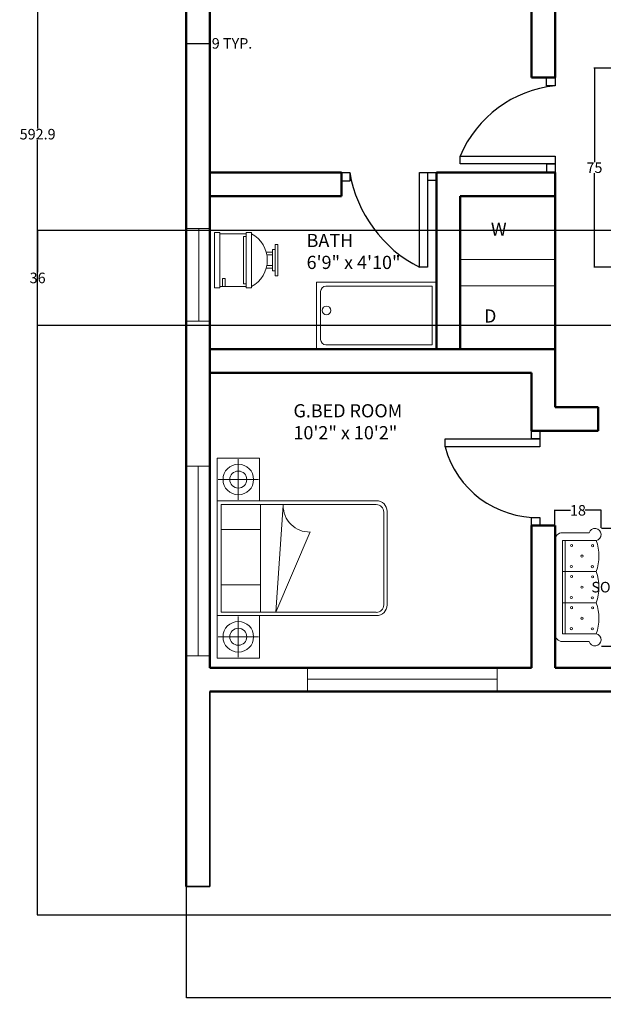
# Model space of a CAD drawing. Units: inches. Extents: x 870 to 1431, y 383 to 1070.
# Tile 1 of 9: x 870 to 1091, y 383 to 756. Entities that reach past the tile are written whole.
import ezdxf

# ---------------------------------------------------------------- set-up
doc = ezdxf.new("R2010")
doc.units = ezdxf.units.IN
doc.header["$MEASUREMENT"] = 0
for name, color, linetype, lineweight in [('A-ANNO-DIMS', 2, 'Continuous', 18), ('A-ANNO-TEXT', 7, 'Continuous', 18), ('A-AREA-IDEN', 7, 'Continuous', 25), ('A-DOOR', 3, 'Continuous', 25), ('A-EQPM', 8, 'Continuous', 20), ('A-FLOR-EXTR', 7, 'Continuous', 35), ('A-FLOR-FIXT', 9, 'Continuous', 18), ('A-FURN', 8, 'Continuous', 18), ('A-GLAZ', 4, 'Continuous', 18), ('A-WALL', 7, 'Continuous', 50)]:
    doc.layers.add(name, color=color, linetype=linetype, lineweight=lineweight)
doc.styles.get("Standard").update_dxf_attribs({"font": 'arial.ttf'})
doc.dimstyles.get("Standard").update_dxf_attribs({"dimtxt": 4, "dimasz": 0.18, "dimexe": 0.18, "dimexo": 0.0625, "dimgap": 0.09, "dimtad": 0, "dimtih": 1, "dimtoh": 1, "dimdec": 0, "dimrnd": 6, "dimzin": 0, "dimdsep": 46, "dimlunit": 3, "dimtxsty": 'Standard', "dimcen": 0.09, "dimadec": 0, "dimazin": 0, "dimtfac": 1, "dimtdec": 0, "dimtofl": 0, "dimtmove": 0, "dimatfit": 3, "dimfxl": 1, "dimtolj": 1, "dimtzin": 0, "dimarcsym": 0})

# ---------------------------------------------------------------- blocks, each defined once
blk = doc.blocks.new('A$C65997121')
for p, q in [((0, 1.5, -0.169), (0, 2, -0.169)), ((0, 2, -0.169), (0.5, 2, -0.169)), ((0, 1.5, -0.169), (0, 2, -0.169)), ((0, 2, -0.169), (0.5, 2, -0.169)), ((0.25, 1.75, -0.169), (0.25, 1.988, -0.169)), ((0.5, 2, -0.169), (1.755, 2, -0.169)), ((0.5, 2, -0.169), (1.512, 2, -0.169)), ((0.5, 2, -0.169), (1.512, 2, -0.169)), ((0.5, 0.125, -0.169), (0.5, 2, -0.169)), ((0.5, 2, -0.169), (0.5, 1.5, -0.169)), ((1.512, 2, -0.169), (2.35, 2, -0.169)), ((1.512, 2, -0.169), (2.35, 2, -0.169)), ((1.85, 2, -0.169), (2.35, 2, -0.169)), ((1.85, 1.5, -0.169), (1.85, 2, -0.169)), ((2.1, 1.75, -0.169), (2.1, 1.988, -0.169)), ((2.35, 2, -0.169), (2.35, 1.5, -0.169)), ((2.35, 2, -0.169), (2.35, 1.5, -0.169)), ((2.35, 2, -0.169), (2.35, 1.5, -0.169)), ((0.538, 1.488, -0.169), (0.538, 1.952, -0.169)), ((0.538, 1.952, -0.169), (1.805, 1.952, -0.169)), ((0.86, 1.952, -0.169), (0.86, 1.488, -0.169)), ((1.512, 1.952, -0.169), (1.512, 1.488, -0.169)), ((1.805, 1.952, -0.169), (1.805, 1.488, -0.169)), ((0.25, 1.75, -0.169), (0.012, 1.75, -0.169)), ((0.25, 1.75, -0.169), (0.25, 1.512, -0.169)), ((0.25, 1.75, -0.169), (0.488, 1.75, -0.169)), ((2.1, 1.75, -0.169), (1.862, 1.75, -0.169)), ((2.1, 1.75, -0.169), (2.338, 1.75, -0.169)), ((2.1, 1.75, -0.169), (2.1, 1.512, -0.169)), ((0.5, 1.5, -0.169), (0, 1.5, -0.169)), ((0.5, 1.5, -0.169), (0, 1.5, -0.169)), ((0.5, 0.125, -0.169), (0.5, 1.5, -0.169)), ((1.805, 1.488, -0.169), (0.538, 1.488, -0.169)), ((0.538, 0.128, -0.169), (0.538, 1.488, -0.169)), ((1.805, 1.488, -0.169), (1.805, 0.128, -0.169)), ((2.35, 1.5, -0.169), (1.85, 1.5, -0.169)), ((2.35, 1.5, -0.169), (1.85, 1.5, -0.169)), ((1.85, 1.5, -0.169), (1.85, 0.125, -0.169)), ((2.35, 1.5, -0.169), (1.85, 1.5, -0.169)), ((1.85, 1.5, -0.169), (1.85, 0.125, -0.169)), ((1.483, 0.905, -0.506), (0.538, 1.31, -0.506)), ((0.538, 1.31, -0.506), (1.797, 1.222, -0.506)), ((1.717, 0.04, -0.169), (0.625, 0.04, -0.169)), ((1.725, 0, -0.169), (0.625, 0, -0.169)), ((1.725, 0, -0.169), (0.625, 0, -0.169))]:
    blk.add_line(p, q)
for centre, radius in [((0.25, 1.75, -0.169), 0.18), ((2.1, 1.75, -0.169), 0.18), ((0.25, 1.75, -0.169), 0.1), ((2.1, 1.75, -0.169), 0.1)]:
    blk.add_circle(centre, radius)
for centre, radius, start, end in [((1.793, 0.911, -0.506), 0.311, 89.3268, 181.1229), ((0.625, 0.125, -0.169), 0.125, 179.9939, 269.9939), ((0.625, 0.125, -0.169), 0.125, 179.9939, 269.9939), ((0.625, 0.128, -0.169), 0.0875, 179.9939, 269.9939), ((1.717, 0.128, -0.169), 0.0875, 269.9939, 359.9939), ((1.725, 0.125, -0.169), 0.125, 269.9939, 359.9939), ((1.725, 0.125, -0.169), 0.125, 269.9939, 359.9939)]:
    blk.add_arc(centre, radius, start, end)
blk = doc.blocks.new('A$C4BF50411')
for p, q in [((0.23, 0.89, -342.513), (2.03, 0.89, -342.513)), ((0.08, 0.74, -342.513), (0.08, 0.228, -342.513)), ((0.23, 0.09, -342.513), (0.23, 0.74, -342.513)), ((0.23, 0.74, -342.513), (2.03, 0.74, -342.513)), ((0.23, 0.69, -342.513), (2.03, 0.69, -342.513)), ((0.83, 0.09, -342.513), (0.83, 0.74, -342.513)), ((1.43, 0.74, -342.513), (1.43, 0.09, -342.513)), ((2.03, 0.74, -342.513), (2.03, 0.09, -342.513)), ((2.18, 0.74, -342.513), (2.18, 0.228, -342.513))]:
    blk.add_line(p, q)
for centre in [(0.33, 0.57, -342.513), (0.735, 0.565, -342.513), (0.93, 0.57, -342.513), (1.335, 0.565, -342.513), (1.53, 0.57, -342.513), (1.935, 0.565, -342.513), (0.53, 0.365, -342.513), (1.13, 0.365, -342.513), (1.73, 0.365, -342.513), (0.325, 0.165, -342.513), (0.73, 0.16, -342.513), (0.925, 0.165, -342.513), (1.33, 0.16, -342.513), (1.525, 0.165, -342.513), (1.93, 0.16, -342.513)]:
    blk.add_circle(centre, 0.02)
for centre, radius, start, end in [((0.23, 0.74, -342.513), 0.15, 90, 180), ((2.03, 0.74, -342.513), 0.15, 0, 90), ((0.115, 0.115, -342.513), 0.118, 107.205, 347.5934), ((2.145, 0.115, -342.513), 0.118, 192.4066, 72.795), ((0.53, 0.938, -342.513), 0.9, 250.5288, 289.4712), ((1.13, 0.938, -342.513), 0.9, 250.5288, 289.4712), ((1.73, 0.938, -342.513), 0.9, 250.5288, 289.4712)]:
    blk.add_arc(centre, radius, start, end)
blk = doc.blocks.new('Toilet - Imperial')
for p, q in [((-10, 22), (-10, 12)), ((-10, 21), (-7, 21)), ((-7, 20), (-10, 20)), ((-7, 21), (-7, 20)), ((10, 12), (10, 22)), ((10.5, 12), (-10.5, 12)), ((-10.5, 10), (-10.5, 12)), ((9, 13), (-9, 13)), ((-9, 13), (-9, 12)), ((9, 12), (9, 13)), ((10.5, 12), (10.5, 10)), ((10.5, 10), (-10.5, 10)), ((-3, 4.4065), (-3, 2)), ((-2, 2), (-2, 4.1658)), ((2, 4.1658), (2, 2)), ((3, 2), (3, 4.4065)), ((4, 2), (-4, 2)), ((-4, 2), (-4, 1)), ((4, 1), (4, 2))]:
    blk.add_line(p, q)
for points in [[(10.5, 22), (10.5, 24), (-10.5, 24), (-10.5, 22)], [(6, 0), (6, 1), (-6, 1), (-6, 0)]]:
    blk.add_lwpolyline(points, close=True)
blk.add_arc((0, 15.3333), 11.3333, 208.0725, 331.9275)
blk = doc.blocks.new('WIN-72IN')
blk.add_line((4.72, 72), (4.72, 0))
blk.add_lwpolyline([(0, 72), (9, 72), (9, 0), (0, 0)], close=True)
blk = doc.blocks.new('WIN-BATH-35IN')
blk.add_line((4.73, 35.25), (4.73, 0))
blk.add_lwpolyline([(0, 0), (0, 35.25), (9, 35.25), (9, 0)], close=True)
blk = doc.blocks.new('*D106')
at = {"layer": 'A-ANNO-DIMS', "color": 0, "lineweight": -2, "transparency": 16777216}
for p, q in [((932.74, 758.23), (932.74, 747.31)), ((941.74, 758.23), (941.74, 747.31)), ((932.92, 747.49), (941.56, 747.49)), ((941.74, 747.49), (941.92, 747.49))]:
    blk.add_line(p, q, dxfattribs=at)
at = {"layer": 'A-ANNO-DIMS', "color": 0, "transparency": 16777216}
for points in [[(932.92, 747.52), (932.92, 747.46), (932.74, 747.49)], [(941.56, 747.52), (941.56, 747.46), (941.74, 747.49)]]:
    blk.add_solid(points, dxfattribs=at)
at = {"layer": 'Defpoints', "color": 0, "transparency": 16777216}
for p in [(932.74, 758.29), (941.74, 758.29), (941.74, 747.49)]:
    blk.add_point(p, dxfattribs=at)
at = {"layer": 'A-ANNO-DIMS', "color": 0, "transparency": 16777216, "insert": (950.19, 747.49), "char_height": 4, "attachment_point": 5}
blk.add_mtext('\\A1;9 TYP.', dxfattribs=at)
blk = doc.blocks.new('*D115')
at = {"layer": 'A-ANNO-DIMS', "color": 0, "lineweight": -2, "transparency": 16777216}
for p, q in [((1090.35, 563.55), (1097.19, 563.55)), ((1097.01, 563.37), (1097.01, 543.29)), ((1097.01, 518.89), (1097.01, 538.97)), ((1090.35, 518.71), (1097.19, 518.71))]:
    blk.add_line(p, q, dxfattribs=at)
at = {"layer": 'A-ANNO-DIMS', "color": 0, "transparency": 16777216}
for points in [[(1096.98, 563.37), (1097.04, 563.37), (1097.01, 563.55)], [(1096.98, 518.89), (1097.04, 518.89), (1097.01, 518.71)]]:
    blk.add_solid(points, dxfattribs=at)
at = {"layer": 'Defpoints', "color": 0, "transparency": 16777216}
for p in [(1090.29, 563.55), (1097.01, 563.55), (1090.29, 518.71)]:
    blk.add_point(p, dxfattribs=at)
at = {"layer": 'A-ANNO-DIMS', "color": 0, "transparency": 16777216, "insert": (1097.01, 541.13), "char_height": 4, "attachment_point": 5}
blk.add_mtext('\\A1;SOFA 45', dxfattribs=at)
blk = doc.blocks.new('*D116')
at = {"layer": 'A-ANNO-DIMS', "color": 0, "lineweight": -2, "transparency": 16777216}
for p, q in [((1072.67, 563.61), (1072.67, 570.46)), ((1072.85, 570.28), (1078.71, 570.28)), ((1090.11, 570.28), (1084.25, 570.28)), ((1090.29, 563.61), (1090.29, 570.46))]:
    blk.add_line(p, q, dxfattribs=at)
at = {"layer": 'A-ANNO-DIMS', "color": 0, "transparency": 16777216}
for points in [[(1072.85, 570.31), (1072.85, 570.25), (1072.67, 570.28)], [(1090.11, 570.31), (1090.11, 570.25), (1090.29, 570.28)]]:
    blk.add_solid(points, dxfattribs=at)
at = {"layer": 'Defpoints', "color": 0, "transparency": 16777216}
for p in [(1072.67, 570.28), (1072.67, 563.55), (1090.29, 563.55)]:
    blk.add_point(p, dxfattribs=at)
at = {"layer": 'A-ANNO-DIMS', "color": 0, "transparency": 16777216, "insert": (1081.48, 570.28), "char_height": 4, "attachment_point": 5}
blk.add_mtext('\\A1;18', dxfattribs=at)
blk = doc.blocks.new('*D124')
at = {"layer": 'A-ANNO-DIMS', "color": 0, "lineweight": -2, "transparency": 16777216}
for p, q in [((1104.9, 738.04), (1087.56, 738.04)), ((1087.74, 737.86), (1087.74, 702.44)), ((1087.74, 662.77), (1087.74, 698.19)), ((1104.9, 662.59), (1087.56, 662.59))]:
    blk.add_line(p, q, dxfattribs=at)
at = {"layer": 'A-ANNO-DIMS', "color": 0, "transparency": 16777216}
for points in [[(1087.71, 737.86), (1087.77, 737.86), (1087.74, 738.04)], [(1087.71, 662.77), (1087.77, 662.77), (1087.74, 662.59)]]:
    blk.add_solid(points, dxfattribs=at)
at = {"layer": 'Defpoints', "color": 0, "transparency": 16777216}
for p in [(1087.74, 738.04), (1104.97, 738.04), (1104.97, 662.59)]:
    blk.add_point(p, dxfattribs=at)
at = {"layer": 'A-ANNO-DIMS', "color": 0, "transparency": 16777216, "insert": (1087.74, 700.32), "char_height": 4, "attachment_point": 5}
blk.add_mtext('\\A1;75', dxfattribs=at)
blk = doc.blocks.new('*D125')
at = {"layer": 'A-ANNO-DIMS', "color": 0, "lineweight": -2, "transparency": 16777216}
for p, q in [((1391.79, 463.41), (1391.79, 385.26)), ((932.79, 427.41), (932.79, 385.26)), ((932.97, 385.44), (1157.7, 385.44)), ((1391.61, 385.44), (1166.88, 385.44))]:
    blk.add_line(p, q, dxfattribs=at)
at = {"layer": 'A-ANNO-DIMS', "color": 0, "transparency": 16777216}
for points in [[(932.97, 385.47), (932.97, 385.41), (932.79, 385.44)], [(1391.61, 385.47), (1391.61, 385.41), (1391.79, 385.44)]]:
    blk.add_solid(points, dxfattribs=at)
at = {"layer": 'Defpoints', "color": 0, "transparency": 16777216}
for p in [(1391.79, 463.48), (932.79, 427.48), (1391.79, 385.44)]:
    blk.add_point(p, dxfattribs=at)
at = {"layer": 'A-ANNO-DIMS', "color": 0, "transparency": 16777216, "insert": (1162.29, 385.44), "char_height": 4, "attachment_point": 5}
blk.add_mtext('\\A1;459', dxfattribs=at)
blk = doc.blocks.new('*D126')
at = {"layer": 'A-ANNO-DIMS', "color": 0, "lineweight": -2, "transparency": 16777216}
for p, q in [((1168.73, 1009.48), (876.24, 1009.48)), ((876.42, 1009.3), (876.42, 715.17)), ((876.42, 416.77), (876.42, 710.9)), ((1094.63, 416.59), (876.24, 416.59))]:
    blk.add_line(p, q, dxfattribs=at)
at = {"layer": 'A-ANNO-DIMS', "color": 0, "transparency": 16777216}
for points in [[(876.39, 1009.3), (876.45, 1009.3), (876.42, 1009.48)], [(876.39, 416.77), (876.45, 416.77), (876.42, 416.59)]]:
    blk.add_solid(points, dxfattribs=at)
at = {"layer": 'Defpoints', "color": 0, "transparency": 16777216}
for p in [(876.42, 1009.48), (1168.79, 1009.48), (1094.7, 416.59)]:
    blk.add_point(p, dxfattribs=at)
at = {"layer": 'A-ANNO-DIMS', "color": 0, "transparency": 16777216, "insert": (876.42, 713.03), "char_height": 4, "attachment_point": 5}
blk.add_mtext('\\A1;592.9', dxfattribs=at)
blk = doc.blocks.new('*D140')
at = {"layer": 'A-ANNO-DIMS', "color": 0, "lineweight": -2, "transparency": 16777216}
for p, q in [((1253.73, 676.48), (876.24, 676.48)), ((876.42, 676.3), (876.42, 660.61)), ((876.42, 640.66), (876.42, 656.34)), ((1253.73, 640.48), (876.24, 640.48))]:
    blk.add_line(p, q, dxfattribs=at)
at = {"layer": 'A-ANNO-DIMS', "color": 0, "transparency": 16777216}
for points in [[(876.39, 676.3), (876.45, 676.3), (876.42, 676.48)], [(876.39, 640.66), (876.45, 640.66), (876.42, 640.48)]]:
    blk.add_solid(points, dxfattribs=at)
at = {"layer": 'Defpoints', "color": 0, "transparency": 16777216}
for p in [(876.42, 676.48), (1253.79, 676.48), (1253.79, 640.48)]:
    blk.add_point(p, dxfattribs=at)
at = {"layer": 'A-ANNO-DIMS', "color": 0, "transparency": 16777216, "insert": (876.42, 658.48), "char_height": 4, "attachment_point": 5}
blk.add_mtext('\\A1;36', dxfattribs=at)

msp = doc.modelspace()

# ---------------------------------------------------------------- linework, layer by layer
at = {"layer": 'A-DOOR'}
for points in [[(1072.8125, 731.3661), (1069.5431, 731.3661), (1069.5431, 734.4675), (1072.8125, 734.4675)], [(1036.7907, 704.7466), (1072.7907, 704.7466), (1072.7907, 701.7466), (1036.7907, 701.7466)], [(1072.7907, 701.7466), (1072.7907, 698.4772), (1069.6894, 698.4772), (1069.6894, 701.7466)], [(991.7907, 695.2078), (991.7907, 698.4772), (994.8921, 698.4772), (994.8921, 695.2078)], [(1024.3348, 698.5023), (1024.3348, 662.5023), (1021.3348, 662.5023), (1021.3348, 698.5023)], [(1027.7898, 695.3895), (1024.5204, 695.3895), (1024.5204, 698.4908), (1027.7898, 698.4908)], [(1067.0637, 597.3823), (1063.7943, 597.3823), (1063.7943, 600.4836), (1067.0637, 600.4836)], [(1031.0637, 597.3823), (1067.0637, 597.3823), (1067.0637, 594.3823), (1031.0637, 594.3823)], [(1067.0601, 564.4772), (1063.7907, 564.4772), (1063.7907, 567.5786), (1067.0601, 567.5786)]]:
    msp.add_lwpolyline(points, close=True, dxfattribs=at)
for centre, radius, start, end in [((1077.1948, 687.7538), 43.832, 95.738003, 157.189718), ((1043.797, 706.7183), 49.5944, 189.565192, 243.069018), ((1065.9432, 603.6513), 36.0901, 194.882073, 271.773498)]:
    msp.add_arc(centre, radius, start, end, dxfattribs=at)
at = {"layer": 'A-EQPM'}
for p, q in [((1036.7907, 665.4772), (1072.7907, 665.4772)), ((1036.7907, 655.4772), (1072.7907, 655.4772))]:
    msp.add_line(p, q, dxfattribs=at)
at = {"layer": 'A-FLOR-EXTR'}
for p in [(941.7907, 501.4772), (932.7907, 427.4772)]:
    msp.add_line(p, (941.7907, 427.4772), dxfattribs=at)
at = {"layer": 'A-FLOR-FIXT'}
msp.add_lwpolyline([(982.2053, 656.9279), (1027.7907, 656.9279), (1027.7907, 631.4772), (982.2053, 631.4772)], close=True, dxfattribs=at)
msp.add_lwpolyline([(985.8053, 655.3279), (1026.1907, 655.3279), (1026.1907, 633.0772), (985.8053, 633.0772, -0.41421356), (983.8053, 635.0772), (983.8053, 653.3279, -0.41421356)], format="xyb", close=True, dxfattribs=at)
msp.add_circle((986.0581, 646.1601), 1.6482, dxfattribs=at)
at = {"layer": 'A-WALL'}
for p, q in [((932.7907, 952.4772), (932.7907, 427.4772)), ((1063.7907, 916.4772), (1063.7907, 734.4772)), ((941.7907, 907.4772), (941.7907, 510.4772)), ((1072.7907, 907.4772), (1072.7907, 734.4772)), ((1063.7907, 734.4772), (1072.7907, 734.4772)), ((941.7907, 698.4772), (991.7907, 698.4772)), ((991.7907, 698.4772), (991.7907, 689.4772)), ((1027.7907, 698.4772), (1027.7907, 631.4772)), ((1027.7907, 698.4772), (1072.7907, 698.4772)), ((1072.7907, 698.4772), (1072.7907, 631.4772)), ((941.7907, 689.4772), (991.7907, 689.4772)), ((1036.7907, 689.4772), (1036.7907, 631.4772)), ((1036.7907, 689.4772), (1072.7907, 689.4772)), ((941.7907, 631.4772), (1072.7907, 631.4772)), ((1072.7907, 631.4772), (1072.7907, 609.4772)), ((941.7907, 622.4772), (1063.7907, 622.4772)), ((1063.7907, 622.4772), (1063.7907, 600.4772)), ((1072.7907, 609.4772), (1089.141, 609.4772)), ((1089.141, 609.4772), (1089.141, 600.4772)), ((1063.7907, 600.4772), (1089.141, 600.4772)), ((1063.7907, 564.4772), (1072.7907, 564.4772)), ((1063.7907, 564.4772), (1063.7907, 510.4772)), ((1072.7907, 564.4772), (1072.7907, 510.4772)), ((941.7907, 510.4772), (1063.7907, 510.4772)), ((1072.7907, 510.4772), (1110.7907, 510.4772)), ((941.7907, 501.4772), (1110.7907, 501.4772))]:
    msp.add_line(p, q, dxfattribs=at)

# ---------------------------------------------------------------- block references
at = {"layer": 'A-FLOR-FIXT', "rotation": 90}
msp.add_blockref('Toilet - Imperial', (967.5715, 665.2213), dxfattribs=at)
at = {"layer": 'A-FURN'}
for name, p, xscale, yscale, zscale, rotation in [('A$C65997121', (1009.0486, 514.215, 5.4452), 32.26790700275002, 32.26790700275002, 32.26790700275002, 90.00000000000078), ('A$C4BF50411', (1090.1847, 518.8869, 6740.5999), 19.67982129011681, 19.67982129011681, 19.67982129011681, 90)]:
    msp.add_blockref(name, p, dxfattribs=dict(at, xscale=xscale, yscale=yscale, zscale=zscale, rotation=rotation))
at = {"layer": 'A-GLAZ'}
for name, p in [('WIN-BATH-35IN', (932.837, 642.041)), ('WIN-72IN', (932.5737, 515.0484))]:
    msp.add_blockref(name, p, dxfattribs=at)
at = {"layer": 'A-GLAZ', "rotation": 89.99999999999969}
msp.add_blockref('WIN-72IN', (1050.8632, 501.5412), dxfattribs=at)

# ---------------------------------------------------------------- texts
at = {"layer": 'A-ANNO-TEXT', "char_height": 5, "attachment_point": 1}
for s, insert in [('W', (1048.4269, 679.4837)), ('D', (1045.8341, 646.5303))]:
    msp.add_mtext_dynamic_manual_height_columns(s, width=69.132678, gutter_width=1, heights=[0], dxfattribs=dict(at, insert=insert))
at = {"layer": 'A-AREA-IDEN', "char_height": 5, "attachment_point": 1}
for s, insert in [('BATH\\P6\'9" x 4\'10"', (978.489, 675.205)), ('G.BED ROOM\\P10\'2" x 10\'2"', (973.5005, 610.5676))]:
    msp.add_mtext_dynamic_manual_height_columns(s, width=69.132678, gutter_width=1, heights=[0], dxfattribs=dict(at, insert=insert))

# ---------------------------------------------------------------- dimensions: what is measured, and where the dimension line sits
at = {"layer": 'A-ANNO-DIMS'}
for base, p1, p2, angle, override, picture, middle in [((876.4215, 1009.4772), (1094.6967, 416.59), (1168.7907, 1009.4772), 90, {"dimdec": 1, "dimlfac": 1, "dimrnd": 0, "dimzin": 0, "dimdsep": 46, "dimlunit": 2}, '*D126', (876.4215, 713.0336)), ((1087.7437, 738.0387), (1104.9659, 662.594), (1104.9659, 738.0387), 90, {"dimdec": 0, "dimlfac": 1, "dimrnd": 0, "dimzin": 0, "dimdsep": 46, "dimlunit": 2}, '*D124', (1087.7437, 700.3164)), ((876.4215, 676.4772), (1253.7907, 640.4772), (1253.7907, 676.4772), 90, {"dimdec": 0, "dimlfac": 1, "dimrnd": 0, "dimzin": 0, "dimdsep": 46, "dimlunit": 2}, '*D140', (876.4215, 658.4772)), ((1072.6748, 570.277), (1090.2878, 563.5502), (1072.6748, 563.5502), 180, {"dimdec": 0, "dimlfac": 1, "dimrnd": 0, "dimzin": 0, "dimdsep": 46, "dimlunit": 2}, '*D116', (1081.4813, 570.277))]:
    dim = msp.add_linear_dim(base=base, p1=p1, p2=p2, angle=angle, dimstyle='Standard', override=override, dxfattribs=at)
    dim.commit()
    dim.dimension.update_dxf_attribs({"geometry": picture, "text_midpoint": middle})
dim = msp.add_linear_dim(base=(941.7363, 747.4949), p1=(932.7363, 758.2949), p2=(941.7363, 758.2949), text='<> TYP.', dimstyle='Standard', override={"dimdec": 0, "dimlfac": 1, "dimrnd": 0, "dimzin": 0, "dimdsep": 46, "dimlunit": 2}, dxfattribs=at)
dim.commit()
dim.dimension.update_dxf_attribs({"geometry": '*D106', "text_midpoint": (950.1878, 747.4949)})
dim = msp.add_linear_dim(base=(1097.0146, 563.5502), p1=(1090.2878, 518.7052), p2=(1090.2878, 563.5502), angle=90, text='SOFA <>', dimstyle='Standard', override={"dimdec": 0, "dimlfac": 1, "dimrnd": 0, "dimzin": 0, "dimdsep": 46, "dimlunit": 2}, dxfattribs=at)
dim.commit()
dim.dimension.update_dxf_attribs({"geometry": '*D115', "text_midpoint": (1097.0146, 541.1277)})
dim = msp.add_linear_dim(base=(1391.7907, 385.44), p1=(932.7907, 427.4772), p2=(1391.7907, 463.4772), dimstyle='Standard', override={"dimdec": 0, "dimlfac": 1, "dimrnd": 0, "dimzin": 0, "dimdsep": 46, "dimlunit": 2}, dxfattribs=at)
dim.commit()
dim.dimension.update_dxf_attribs({"geometry": '*D125', "text_midpoint": (1162.2907, 385.44)})

doc.saveas('drawing.dxf')
